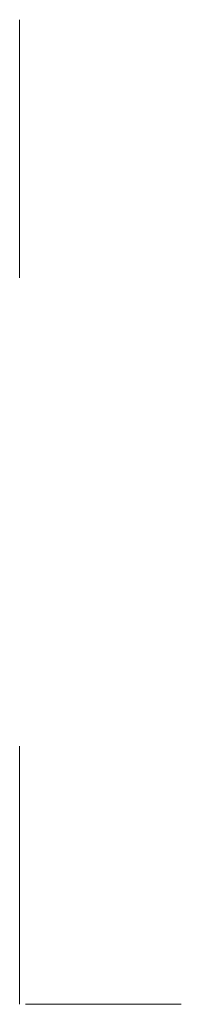
# Model space of a CAD drawing. Units: millimetres. Extents: x 160 to 187, y 283 to 447.
import ezdxf

# ---------------------------------------------------------------- set-up
doc = ezdxf.new("R2010")
doc.units = ezdxf.units.MM
doc.layers.add('M-CONS', color=8, linetype='Continuous', lineweight=13)

msp = doc.modelspace()

# ---------------------------------------------------------------- linework, layer by layer
at = {"layer": 'M-CONS'}
for p, q in [((160.45, 404.24, 47.62), (160.45, 447.25, 12)), ((160.45, 326.27, 47.62), (160.45, 283.25, 12)), ((161.45, 283.25), (161.45, 283.25, 3)), ((161.45, 283.25, 3), (187.45, 283.25, 3)), ((187.45, 283.25, 3), (187.45, 283.25))]:
    msp.add_line(p, q, dxfattribs=at)

doc.saveas('drawing.dxf')
